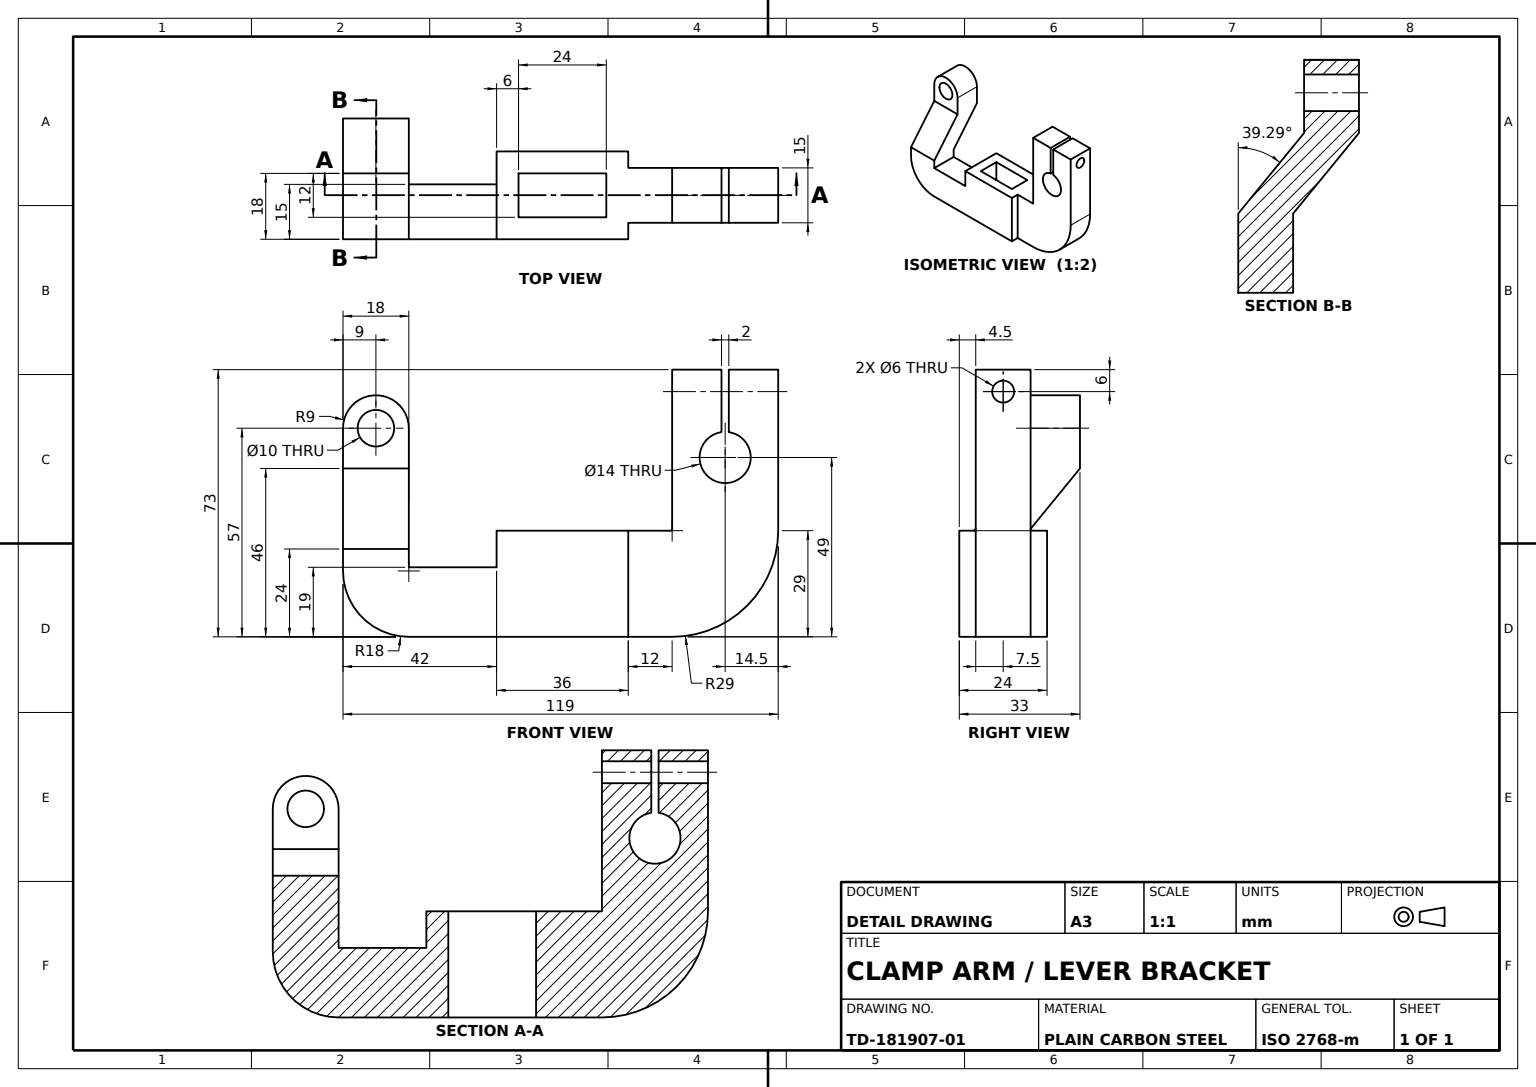
from build123d import *

# Parameters (mm, degrees)
Z_PROFILE_PLATE_DEPTH       = 15
ARM_EXTENSION_BOSS_DEPTH    = 24
CLAMP_START                 = -4.5
CLAMP_HUB_BOSS_DEPTH        = 15
CENTER_BLOCK_DEPTH          = 18
PIVOT_START                 = -1.5
PIVOT_LUG_DEPTH             = 7.5
PIVOT_HOLE_SKETCH_R         = 5
PIVOT_HOLE_10_DEPTH         = 15
RECTANGULAR_POCKET_SKETCH_W = 24
RECTANGULAR_POCKET_SKETCH_H = 12
RECTANGULAR_POCKET_DEPTH    = 116.004347744
CLAMP_SLOT_DEPTH            = 15
CLAMP_SCREW_HOLE_SKETCH_R   = 3
CLAMP_SCREW_HOLE_6_DEPTH    = 121.490663539


with BuildPart() as part:
    # Z Profile Sketch → Z Profile Plate (new body)
    with BuildSketch(Plane.XY):
        with BuildLine():
            ThreePointArc((-18, 18), (-12.727922061, 5.272077939), (0, 0))
            Line((0, 0), (24, 0))
            Line((24, 0), (24, 19))
            Line((24, 19), (0, 19))
            Line((0, 19), (0, 24))
            Line((0, 24), (-16.970562748, 24))
            Line((-16.970562748, 24), (-18, 24))
            Line((-18, 24), (-18, 18))
        make_face()
    extrude(amount=-Z_PROFILE_PLATE_DEPTH)

    # Sketch1_6 → Arm Extension Boss (add)
    with BuildSketch(Plane.XY):
        Polygon((24, 19), (24, 0), (60, 0), (60, 29), (24, 29), align=None)
    extrude(amount=-ARM_EXTENSION_BOSS_DEPTH)

    # Sketch1_7 → Clamp Hub Boss (add)
    with BuildSketch(Plane.XY.offset(CLAMP_START)):
        with BuildLine():
            Line((60, 0), (72, 0))
            ThreePointArc((72, 0), (92.506096654, 8.493903346), (101, 29))
            Line((101, 29), (101, 73))
            Line((101, 73), (72, 73))
            Line((72, 73), (72, 29))
            Line((72, 29), (60, 29))
            Line((60, 29), (60, 0))
        make_face()
    extrude(amount=-CLAMP_HUB_BOSS_DEPTH)

    # Center Block Sketch → Center Block (add)
    with BuildSketch(Plane.ZY.offset(18)):
        Polygon((-33, 46), (-15, 24), (0, 24), (-18, 46), align=None)
    extrude(amount=-CENTER_BLOCK_DEPTH)

    # Pivot Lug Sketch → Pivot Lug (add, symmetric)
    with BuildSketch(Plane.XY.offset(-24).offset(PIVOT_START)):
        with BuildLine():
            Line((-18, 57), (-18, 46))
            Line((-18, 46), (0, 46))
            Line((0, 46), (0, 57))
            ThreePointArc((0, 57), (-9, 66), (-18, 57))
        make_face()
    extrude(amount=PIVOT_LUG_DEPTH, both=True)

    # Pivot Hole Sketch → Pivot Hole _10 (cut)
    with BuildSketch(Plane.XY.offset(-18)):
        with Locations((-9, 57)):
            Circle(PIVOT_HOLE_SKETCH_R)
    extrude(amount=-PIVOT_HOLE_10_DEPTH, mode=Mode.SUBTRACT)

    # Rectangular Pocket Sketch → Rectangular Pocket (cut, through all)
    with BuildSketch(Plane(origin=(0, 29, 0), x_dir=(1, 0, 0), z_dir=(0, 1, 0))):
        with Locations((42, 12)):
            Rectangle(RECTANGULAR_POCKET_SKETCH_W, RECTANGULAR_POCKET_SKETCH_H)
    extrude(amount=-RECTANGULAR_POCKET_DEPTH, mode=Mode.SUBTRACT)

    # Clamp Slot Sketch → Clamp Slot (cut)
    with BuildSketch(Plane.XY.offset(-4.5)):
        with BuildLine():
            Line((87.5, 55.92820323), (87.5, 73))
            Line((87.5, 73), (85.5, 73))
            Line((85.5, 73), (85.5, 55.92820323))
            ThreePointArc((85.5, 55.92820323), (86.5, 42), (87.5, 55.92820323))
        make_face()
    extrude(amount=-CLAMP_SLOT_DEPTH, mode=Mode.SUBTRACT)

    # Clamp Screw Hole Sketch → Clamp Screw Hole _6 (cut, through all)
    with BuildSketch(Plane.ZY.offset(-72)):
        with Locations((-12, 67)):
            Circle(CLAMP_SCREW_HOLE_SKETCH_R)
    extrude(amount=-CLAMP_SCREW_HOLE_6_DEPTH, mode=Mode.SUBTRACT)


solid = part.part
